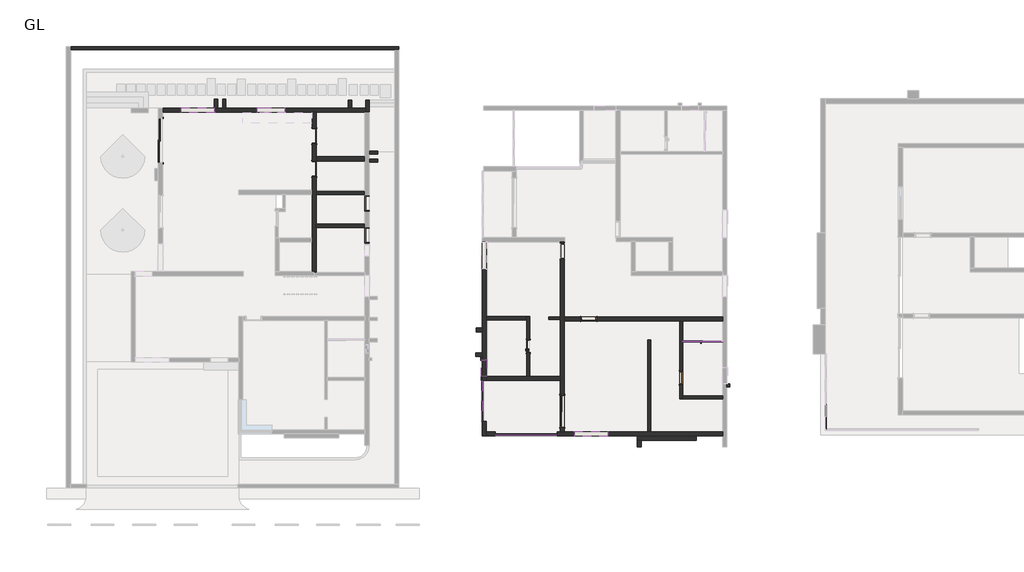
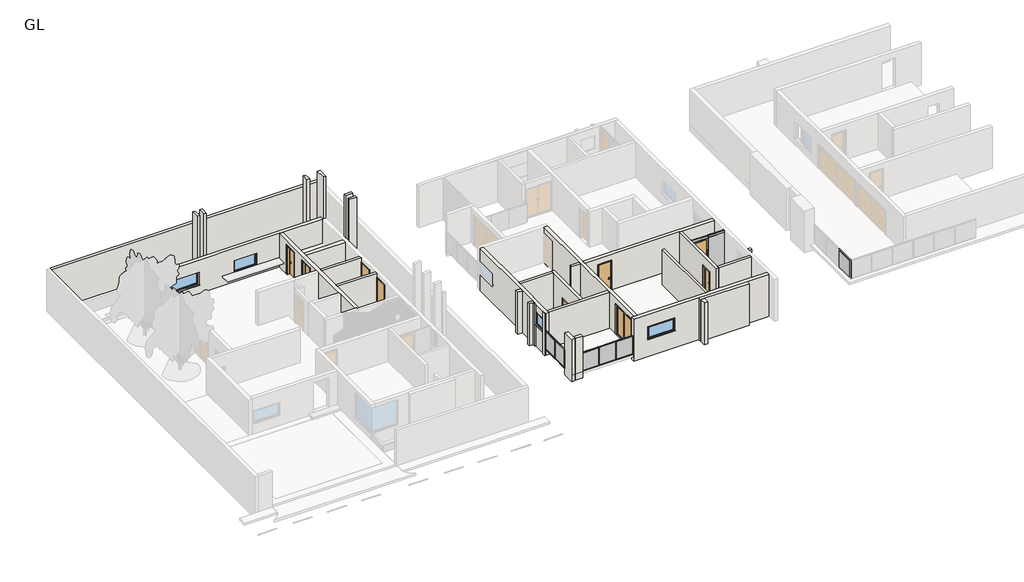
# One storey, part 2 of 6: 32 walls, 26 members, 10 doors, 9 plates, 4 windows.
# Revit data of these elements (continued)
# Elements 47, 48, 49 (IfcWall, "6\" WALL") (continued)
#   Base Offset = 0' - 0"
#   wall height = 9' - 10.11024"
#   Phase Created = New Construction
#   Base Constraint = GL
#   Top Constraint = FFL
#   Materials on its faces: "Brick, Common"
# Elements 50, 51, 52, 58, 59, 60, 61, 62 (IfcWall, "7\" WALL")
#   Top Offset = 0' - 0"
#   Base Offset = 0' - 0"
#   wall height = 9' - 10.11024"
#   Phase Created = New Construction
#   Base Constraint = GL
#   Top Constraint = FFL
#   Materials on its faces: "Brick, Common"
# Elements 53, 54, 55, 56, 57 (IfcWall, "7\" WALL")
#   Top Offset = 0' - 0"
#   Base Offset = 0' - 0"
#   wall height = 19' - 8.22047"
#   Phase Created = New Construction
#   Base Constraint = GL
#   Top Constraint = SFL
#   Materials on its faces: "Brick, Common"
# Elements 63, 64, 65, 66, 67, 68, 69, 70, 71, 72, 73, 74, 75, 76 (IfcWall, "9\" INNER WALL")
#   Top Offset = 0' - 0"
#   Base Offset = 0' - 0"
#   wall height = 9' - 10.11024"
#   Phase Created = New Construction
#   Base Constraint = GL
#   Top Constraint = FFL
#   Materials on its faces: "Brick, Common"
# Element 77 (IfcWall, "9\" INNER WALL 2")
#   Top Offset = 0' - 0"
#   Base Offset = 0' - 0"
#   wall height = 9' - 10.11024"
#   Phase Created = New Construction
#   Base Constraint = GL
#   Top Constraint = FFL
#   Materials on its faces: "Brick, Common"
# Element 78 (IfcWindow, "Windows_Sgl_Plain : 3'")
#   Mark = "17"
#   Phase Created = New Construction
#   Materials on its faces: "Window Frame", "Glass"
# Element 79 (IfcWindow, "Windows_Sgl_Plain : 5'")
#   Mark = "21"
#   Phase Created = New Construction
#   Materials on its faces: "Window Frame", "Glass"
# Element 80 (IfcWindow, "Windows_Sgl_Plain : 6'")
#   Mark = "16"
#   Phase Created = New Construction
#   Materials on its faces: "Window Frame", "Glass"
# Element 81 (IfcWindow, "Windows_Sgl_Plain : 6'")
#   Mark = "22"
#   Phase Created = New Construction
#   Materials on its faces: "Window Frame", "Glass"
# Materials
#   "Puerta - Panel": class "Madera", colour RGB 210 159 95, transparency 0
#   "Door - Handle": colour RGB 0 0 0, transparency 0, Keynote = "P21", Cost = 0
#   "Door - Frame/Mullion (1)": class "Wood", colour RGB 212 179 113, transparency 0, Keynote = "L20", Cost = 0
#   "Door - Panel": class "Wood", colour RGB 210 159 95, transparency 0, Keynote = "L20", Cost = 0
#   "Door - Architrave": class "Wood", colour RGB 154 90 5, transparency 0, Keynote = "P20", Cost = 0
#   "Metal - Aluminum": class "Metal", colour RGB 247 247 247, transparency 0
#   "Glass": class "Glass", colour RGB 0 128 192, transparency 0.9, Description = "Soda Lime Glass", Cost = 0
#   "Brick, Common": class "Masonry", colour RGB 170 100 105, transparency 0, Description = "Common brick", Cost = 0
#   "Window Frame": colour RGB 249 249 249, transparency 0, Keynote = "L10", Cost = 0
#   "Cristal": class "Vidrio", colour RGB 0 0 255, transparency 0.75
#   "Aluminium": class "Metal", colour RGB 247 247 247, transparency 0, Description = "Aluminium 6061", Cost = 0
